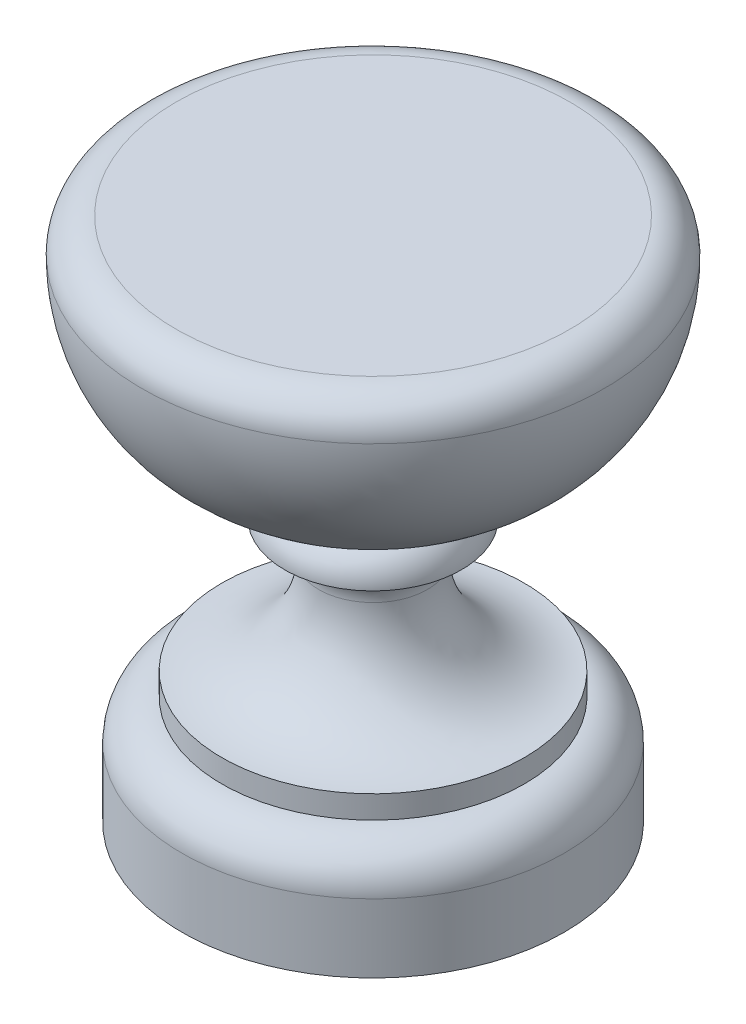
ISO-10303-21;
HEADER;
FILE_DESCRIPTION(('STEP AP214'),'2;1');
FILE_NAME('part.step','',(''),(''),'','','');
FILE_SCHEMA(('AUTOMOTIVE_DESIGN { 1 0 10303 214 1 1 1 1 }'));
ENDSEC;
DATA;
#1=APPLICATION_CONTEXT('core data for automotive mechanical design processes');
#2=APPLICATION_PROTOCOL_DEFINITION('international standard','automotive_design',2000,#1);
#3=PRODUCT_CONTEXT('',#1,'mechanical');
#4=PRODUCT('Part','Part','',(#3));
#5=PRODUCT_RELATED_PRODUCT_CATEGORY('part','',(#4));
#6=PRODUCT_DEFINITION_FORMATION('','',#4);
#7=PRODUCT_DEFINITION_CONTEXT('part definition',#1,'design');
#8=PRODUCT_DEFINITION('design','',#6,#7);
#9=PRODUCT_DEFINITION_SHAPE('','',#8);
#10=(LENGTH_UNIT() NAMED_UNIT(*) SI_UNIT(.MILLI.,.METRE.));
#11=(NAMED_UNIT(*) PLANE_ANGLE_UNIT() SI_UNIT($,.RADIAN.));
#12=(NAMED_UNIT(*) SI_UNIT($,.STERADIAN.) SOLID_ANGLE_UNIT());
#13=UNCERTAINTY_MEASURE_WITH_UNIT(LENGTH_MEASURE(1.E-05),#10,'distance_accuracy_value','');
#14=(GEOMETRIC_REPRESENTATION_CONTEXT(3) GLOBAL_UNCERTAINTY_ASSIGNED_CONTEXT((#13)) GLOBAL_UNIT_ASSIGNED_CONTEXT((#10,
#11,#12)) REPRESENTATION_CONTEXT('',''));
#15=CARTESIAN_POINT('',(0.,0.,0.));
#16=DIRECTION('',(0.,0.,1.));
#17=DIRECTION('',(1.,0.,0.));
#18=AXIS2_PLACEMENT_3D('',#15,#16,#17);
#19=CARTESIAN_POINT('',(0.,0.,0.));
#20=DIRECTION('',(0.,1.,0.));
#21=DIRECTION('',(-1.,0.,0.));
#22=AXIS2_PLACEMENT_3D('',#19,#20,#21);
#23=PLANE('',#22);
#24=CARTESIAN_POINT('',(0.,0.,0.));
#25=DIRECTION('',(0.,1.,0.));
#26=DIRECTION('',(-1.,0.,0.));
#27=AXIS2_PLACEMENT_3D('',#24,#25,#26);
#28=CIRCLE('',#27,33.5);
#29=CARTESIAN_POINT('',(-33.5,0.,0.));
#30=VERTEX_POINT('',#29);
#31=EDGE_CURVE('E10',#30,#30,#28,.T.);
#32=ORIENTED_EDGE('',*,*,#31,.F.);
#33=EDGE_LOOP('',(#32));
#34=FACE_BOUND('',#33,.T.);
#35=ADVANCED_FACE('F40',(#34),#23,.F.);
#36=CARTESIAN_POINT('',(0.,92.,0.));
#37=DIRECTION('',(0.,1.,0.));
#38=DIRECTION('',(-1.,0.,0.));
#39=AXIS2_PLACEMENT_3D('',#36,#37,#38);
#40=CYLINDRICAL_SURFACE('',#39,33.5);
#41=CARTESIAN_POINT('',(0.,12.,0.));
#42=DIRECTION('',(0.,1.,0.));
#43=DIRECTION('',(-1.,0.,0.));
#44=AXIS2_PLACEMENT_3D('',#41,#42,#43);
#45=CIRCLE('',#44,33.5);
#46=CARTESIAN_POINT('',(-33.5,12.,0.));
#47=VERTEX_POINT('',#46);
#48=EDGE_CURVE('E43',#47,#47,#45,.T.);
#49=ORIENTED_EDGE('',*,*,#48,.F.);
#50=EDGE_LOOP('',(#49));
#51=FACE_BOUND('',#50,.T.);
#52=ORIENTED_EDGE('',*,*,#31,.T.);
#53=EDGE_LOOP('',(#52));
#54=FACE_BOUND('',#53,.T.);
#55=ADVANCED_FACE('F121',(#51,#54),#40,.T.);
#56=CARTESIAN_POINT('',(0.,12.,0.));
#57=DIRECTION('',(0.,1.,0.));
#58=DIRECTION('',(-1.,0.,0.));
#59=AXIS2_PLACEMENT_3D('',#56,#57,#58);
#60=TOROIDAL_SURFACE('',#59,26.5,6.99999999999999);
#61=CARTESIAN_POINT('',(0.,19.,0.));
#62=DIRECTION('',(0.,1.,0.));
#63=DIRECTION('',(-1.,0.,0.));
#64=AXIS2_PLACEMENT_3D('',#61,#62,#63);
#65=CIRCLE('',#64,26.5);
#66=CARTESIAN_POINT('',(-26.5,19.,0.));
#67=VERTEX_POINT('',#66);
#68=EDGE_CURVE('E50',#67,#67,#65,.T.);
#69=ORIENTED_EDGE('',*,*,#68,.F.);
#70=EDGE_LOOP('',(#69));
#71=FACE_BOUND('',#70,.T.);
#72=ORIENTED_EDGE('',*,*,#48,.T.);
#73=EDGE_LOOP('',(#72));
#74=FACE_BOUND('',#73,.T.);
#75=ADVANCED_FACE('F117',(#71,#74),#60,.T.);
#76=CARTESIAN_POINT('',(0.,92.,0.));
#77=DIRECTION('',(0.,1.,0.));
#78=DIRECTION('',(-1.,0.,0.));
#79=AXIS2_PLACEMENT_3D('',#76,#77,#78);
#80=CYLINDRICAL_SURFACE('',#79,26.5);
#81=CARTESIAN_POINT('',(0.,23.,0.));
#82=DIRECTION('',(0.,1.,0.));
#83=DIRECTION('',(-1.,0.,0.));
#84=AXIS2_PLACEMENT_3D('',#81,#82,#83);
#85=CIRCLE('',#84,26.5);
#86=CARTESIAN_POINT('',(-26.5,23.,0.));
#87=VERTEX_POINT('',#86);
#88=EDGE_CURVE('E51',#87,#87,#85,.T.);
#89=ORIENTED_EDGE('',*,*,#88,.F.);
#90=EDGE_LOOP('',(#89));
#91=FACE_BOUND('',#90,.T.);
#92=ORIENTED_EDGE('',*,*,#68,.T.);
#93=EDGE_LOOP('',(#92));
#94=FACE_BOUND('',#93,.T.);
#95=ADVANCED_FACE('F109',(#91,#94),#80,.T.);
#96=CARTESIAN_POINT('',(0.,40.,0.));
#97=DIRECTION('',(0.,1.,0.));
#98=DIRECTION('',(-1.,0.,0.));
#99=AXIS2_PLACEMENT_3D('',#96,#97,#98);
#100=TOROIDAL_SURFACE('',#99,26.5,17.);
#101=CARTESIAN_POINT('',(0.,40.,0.));
#102=DIRECTION('',(0.,1.,0.));
#103=DIRECTION('',(-1.,0.,0.));
#104=AXIS2_PLACEMENT_3D('',#101,#102,#103);
#105=CIRCLE('',#104,9.5);
#106=CARTESIAN_POINT('',(-9.5,40.,0.));
#107=VERTEX_POINT('',#106);
#108=EDGE_CURVE('E57',#107,#107,#105,.T.);
#109=ORIENTED_EDGE('',*,*,#108,.F.);
#110=EDGE_LOOP('',(#109));
#111=FACE_BOUND('',#110,.T.);
#112=ORIENTED_EDGE('',*,*,#88,.T.);
#113=EDGE_LOOP('',(#112));
#114=FACE_BOUND('',#113,.T.);
#115=ADVANCED_FACE('F102',(#111,#114),#100,.F.);
#116=CARTESIAN_POINT('',(0.,40.,0.));
#117=DIRECTION('',(0.,1.,0.));
#118=DIRECTION('',(-1.,0.,0.));
#119=AXIS2_PLACEMENT_3D('',#116,#117,#118);
#120=TOROIDAL_SURFACE('',#119,15.5,6.);
#121=CARTESIAN_POINT('',(0.,46.,0.));
#122=DIRECTION('',(0.,1.,0.));
#123=DIRECTION('',(-1.,0.,0.));
#124=AXIS2_PLACEMENT_3D('',#121,#122,#123);
#125=CIRCLE('',#124,15.5);
#126=CARTESIAN_POINT('',(-15.5,46.,0.));
#127=VERTEX_POINT('',#126);
#128=EDGE_CURVE('E56',#127,#127,#125,.T.);
#129=ORIENTED_EDGE('',*,*,#128,.F.);
#130=EDGE_LOOP('',(#129));
#131=FACE_BOUND('',#130,.T.);
#132=ORIENTED_EDGE('',*,*,#108,.T.);
#133=EDGE_LOOP('',(#132));
#134=FACE_BOUND('',#133,.T.);
#135=ADVANCED_FACE('F98',(#131,#134),#120,.F.);
#136=CARTESIAN_POINT('',(0.,46.,0.));
#137=DIRECTION('',(0.,1.,0.));
#138=DIRECTION('',(-1.,0.,0.));
#139=AXIS2_PLACEMENT_3D('',#136,#137,#138);
#140=TOROIDAL_SURFACE('',#139,9.50000000000001,6.);
#141=CARTESIAN_POINT('',(0.,52.,0.));
#142=DIRECTION('',(0.,1.,0.));
#143=DIRECTION('',(-1.,0.,0.));
#144=AXIS2_PLACEMENT_3D('',#141,#142,#143);
#145=CIRCLE('',#144,9.50000000000001);
#146=CARTESIAN_POINT('',(-9.50000000000001,52.,0.));
#147=VERTEX_POINT('',#146);
#148=EDGE_CURVE('E65',#147,#147,#145,.T.);
#149=ORIENTED_EDGE('',*,*,#148,.F.);
#150=EDGE_LOOP('',(#149));
#151=FACE_BOUND('',#150,.T.);
#152=ORIENTED_EDGE('',*,*,#128,.T.);
#153=EDGE_LOOP('',(#152));
#154=FACE_BOUND('',#153,.T.);
#155=ADVANCED_FACE('F95',(#151,#154),#140,.T.);
#156=CARTESIAN_POINT('',(0.,92.,0.));
#157=DIRECTION('',(0.,1.,0.));
#158=DIRECTION('',(-1.,0.,0.));
#159=AXIS2_PLACEMENT_3D('',#156,#157,#158);
#160=CYLINDRICAL_SURFACE('',#159,9.50000000000001);
#161=CARTESIAN_POINT('',(0.,55.,0.));
#162=DIRECTION('',(0.,1.,0.));
#163=DIRECTION('',(-1.,0.,0.));
#164=AXIS2_PLACEMENT_3D('',#161,#162,#163);
#165=CIRCLE('',#164,9.5);
#166=CARTESIAN_POINT('',(-9.5,55.,0.));
#167=VERTEX_POINT('',#166);
#168=EDGE_CURVE('E63',#167,#167,#165,.T.);
#169=ORIENTED_EDGE('',*,*,#168,.F.);
#170=EDGE_LOOP('',(#169));
#171=FACE_BOUND('',#170,.T.);
#172=ORIENTED_EDGE('',*,*,#148,.T.);
#173=EDGE_LOOP('',(#172));
#174=FACE_BOUND('',#173,.T.);
#175=ADVANCED_FACE('F88',(#171,#174),#160,.T.);
#176=CARTESIAN_POINT('',(0.,86.,0.));
#177=DIRECTION('',(0.,1.,0.));
#178=DIRECTION('',(-1.,0.,0.));
#179=AXIS2_PLACEMENT_3D('',#176,#177,#178);
#180=DEGENERATE_TOROIDAL_SURFACE('',#179,9.5,31.,.T.);
#181=CARTESIAN_POINT('',(0.,86.,0.));
#182=DIRECTION('',(0.,1.,0.));
#183=DIRECTION('',(-1.,0.,0.));
#184=AXIS2_PLACEMENT_3D('',#181,#182,#183);
#185=CIRCLE('',#184,40.5);
#186=CARTESIAN_POINT('',(-40.5,86.,0.));
#187=VERTEX_POINT('',#186);
#188=EDGE_CURVE('E68',#187,#187,#185,.T.);
#189=ORIENTED_EDGE('',*,*,#188,.F.);
#190=EDGE_LOOP('',(#189));
#191=FACE_BOUND('',#190,.T.);
#192=ORIENTED_EDGE('',*,*,#168,.T.);
#193=EDGE_LOOP('',(#192));
#194=FACE_BOUND('',#193,.T.);
#195=ADVANCED_FACE('F78',(#191,#194),#180,.T.);
#196=CARTESIAN_POINT('',(0.,86.,0.));
#197=DIRECTION('',(0.,1.,0.));
#198=DIRECTION('',(-1.,0.,0.));
#199=AXIS2_PLACEMENT_3D('',#196,#197,#198);
#200=TOROIDAL_SURFACE('',#199,34.5,6.);
#201=CARTESIAN_POINT('',(0.,92.,0.));
#202=DIRECTION('',(0.,1.,0.));
#203=DIRECTION('',(-1.,0.,0.));
#204=AXIS2_PLACEMENT_3D('',#201,#202,#203);
#205=CIRCLE('',#204,34.5);
#206=CARTESIAN_POINT('',(-34.5,92.,0.));
#207=VERTEX_POINT('',#206);
#208=EDGE_CURVE('E72',#207,#207,#205,.T.);
#209=ORIENTED_EDGE('',*,*,#208,.F.);
#210=EDGE_LOOP('',(#209));
#211=FACE_BOUND('',#210,.T.);
#212=ORIENTED_EDGE('',*,*,#188,.T.);
#213=EDGE_LOOP('',(#212));
#214=FACE_BOUND('',#213,.T.);
#215=ADVANCED_FACE('F80',(#211,#214),#200,.T.);
#216=CARTESIAN_POINT('',(34.5,92.,0.));
#217=DIRECTION('',(0.,-1.,0.));
#218=DIRECTION('',(1.,0.,0.));
#219=AXIS2_PLACEMENT_3D('',#216,#217,#218);
#220=PLANE('',#219);
#221=ORIENTED_EDGE('',*,*,#208,.T.);
#222=EDGE_LOOP('',(#221));
#223=FACE_BOUND('',#222,.T.);
#224=ADVANCED_FACE('F73',(#223),#220,.F.);
#225=CLOSED_SHELL('',(#35,#55,#75,#95,#115,#135,#155,#175,#195,#215,#224));
#226=MANIFOLD_SOLID_BREP('B2',#225);
#227=ADVANCED_BREP_SHAPE_REPRESENTATION('',(#18,#226),#14);
#228=SHAPE_DEFINITION_REPRESENTATION(#9,#227);
ENDSEC;
END-ISO-10303-21;
